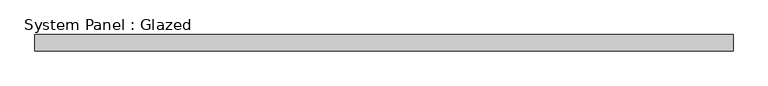
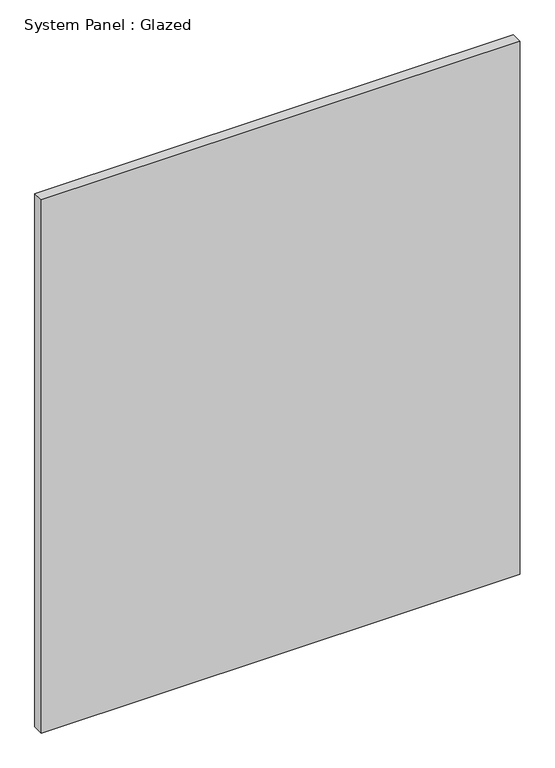
"""IFC4 building model written with IfcOpenShell, lengths in millimetres: plate geometry, System Panel : Glazed."""

from ifc_helpers import new_model, si_unit, origin, origin_with_axes, place, context, project, spatial, polyline, outline, extrude, source, transform, mapped, element, save


def system_panel_glazed_1b898e97(model_context):
    return source(origin(), model_context, "Body", "SweptSolid", [
        extrude(outline(polyline([(549.2750001, 19.05), (-549.2750001, 19.05), (-549.2750001, 44.45), (549.2750001, 44.45), (549.2750001, 19.05)])), origin_with_axes(), (0.0, 0.0, 1.0), 1292.6724956),
    ])


if __name__ == "__main__":
    model = new_model("IFC4")
    model_context = context("Model", 3, world=origin())
    ifc_project = project(units=[si_unit("LENGTHUNIT", "METRE", prefix="MILLI")], contexts=[model_context])
    site = spatial("IfcSite", under=ifc_project)
    building = spatial("IfcBuilding", under=site)
    placement = place(None, origin())
    system_panel_glazed_shape = system_panel_glazed_1b898e97(model_context)
    element("IfcPlate", 1, ObjectType="System Panel : Glazed", at=placement, inside=building, context=model_context, shape_type="MappedRepresentation", body=[
        mapped(system_panel_glazed_shape, transform((0.0, 0.0, 0.0), x_axis=(1.0, 0.0, 0.0), y_axis=(0.0, 1.0, 0.0), z_axis=(0.0, 0.0, 1.0))),
    ])
    save(model, "model.ifc")

# Revit data of these elements
# Type "System Panel : Glazed"
#   Construction Type Id = "GSP4R"
#   Analytic Construction = "1/8 in Pilkington single glazing"
#   Visual Light Transmittance = 0.9
#   Solar Heat Gain Coefficient = 0.86
#   Heat Transfer Coefficient (U) = 1.18115 BTU/(h·ft²·°F)
#   Define Thermal Properties by = 1
# Element 1 (IfcPlate, "System Panel : Glazed")
#   Materials on its faces: "Glass"
# Materials
#   "Glass": class "Glass", colour RGB 0 128 192, transparency 0.75, Description = "Soda Lime Glass", Cost = 0
